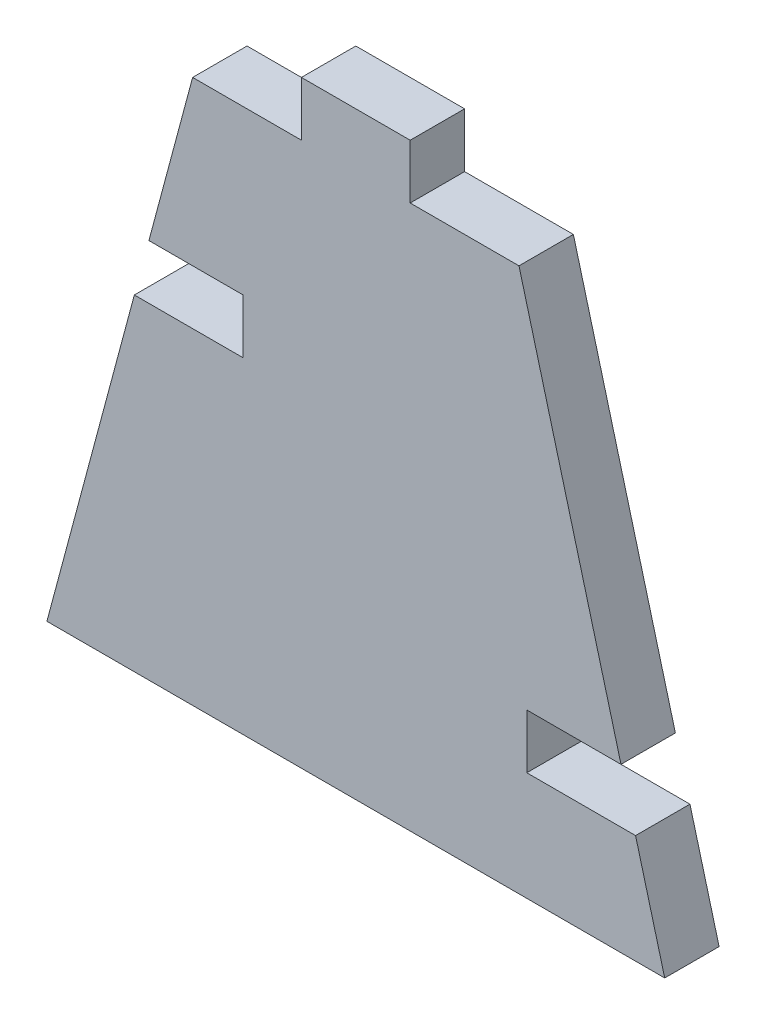
ISO-10303-21;
HEADER;
FILE_DESCRIPTION(('STEP AP214'),'2;1');
FILE_NAME('part.step','',(''),(''),'','','');
FILE_SCHEMA(('AUTOMOTIVE_DESIGN { 1 0 10303 214 1 1 1 1 }'));
ENDSEC;
DATA;
#1=APPLICATION_CONTEXT('core data for automotive mechanical design processes');
#2=APPLICATION_PROTOCOL_DEFINITION('international standard','automotive_design',2000,#1);
#3=PRODUCT_CONTEXT('',#1,'mechanical');
#4=PRODUCT('Part','Part','',(#3));
#5=PRODUCT_RELATED_PRODUCT_CATEGORY('part','',(#4));
#6=PRODUCT_DEFINITION_FORMATION('','',#4);
#7=PRODUCT_DEFINITION_CONTEXT('part definition',#1,'design');
#8=PRODUCT_DEFINITION('design','',#6,#7);
#9=PRODUCT_DEFINITION_SHAPE('','',#8);
#10=(LENGTH_UNIT() NAMED_UNIT(*) SI_UNIT(.MILLI.,.METRE.));
#11=(NAMED_UNIT(*) PLANE_ANGLE_UNIT() SI_UNIT($,.RADIAN.));
#12=(NAMED_UNIT(*) SI_UNIT($,.STERADIAN.) SOLID_ANGLE_UNIT());
#13=UNCERTAINTY_MEASURE_WITH_UNIT(LENGTH_MEASURE(1.E-05),#10,'distance_accuracy_value','');
#14=(GEOMETRIC_REPRESENTATION_CONTEXT(3) GLOBAL_UNCERTAINTY_ASSIGNED_CONTEXT((#13)) GLOBAL_UNIT_ASSIGNED_CONTEXT((#10,
#11,#12)) REPRESENTATION_CONTEXT('',''));
#15=CARTESIAN_POINT('',(0.,0.,0.));
#16=DIRECTION('',(0.,0.,1.));
#17=DIRECTION('',(1.,0.,0.));
#18=AXIS2_PLACEMENT_3D('',#15,#16,#17);
#19=CARTESIAN_POINT('',(0.,0.,5.));
#20=DIRECTION('',(0.965925826289069,-0.258819045102518,0.));
#21=DIRECTION('',(0.258819045102518,0.965925826289069,0.));
#22=AXIS2_PLACEMENT_3D('',#19,#20,#21);
#23=PLANE('',#22);
#24=DIRECTION('',(-0.258819045102518,-0.965925826289069,0.));
#25=VECTOR('',#24,1.);
#26=CARTESIAN_POINT('',(0.,0.,-5.));
#27=LINE('',#26,#25);
#28=CARTESIAN_POINT('',(16.0769515458672,60.,-5.));
#29=VERTEX_POINT('',#28);
#30=CARTESIAN_POINT('',(0.,0.,-5.));
#31=VERTEX_POINT('',#30);
#32=EDGE_CURVE('E181',#29,#31,#27,.T.);
#33=ORIENTED_EDGE('',*,*,#32,.T.);
#34=DIRECTION('',(0.,0.,-1.));
#35=VECTOR('',#34,1.);
#36=CARTESIAN_POINT('',(0.,0.,5.));
#37=LINE('',#36,#35);
#38=CARTESIAN_POINT('',(0.,0.,5.));
#39=VERTEX_POINT('',#38);
#40=EDGE_CURVE('E11',#39,#31,#37,.T.);
#41=ORIENTED_EDGE('',*,*,#40,.F.);
#42=DIRECTION('',(-0.258819045102518,-0.965925826289069,0.));
#43=VECTOR('',#42,1.);
#44=CARTESIAN_POINT('',(0.,0.,5.));
#45=LINE('',#44,#43);
#46=CARTESIAN_POINT('',(16.0769515458672,60.,5.));
#47=VERTEX_POINT('',#46);
#48=EDGE_CURVE('E213',#47,#39,#45,.T.);
#49=ORIENTED_EDGE('',*,*,#48,.F.);
#50=DIRECTION('',(0.,0.,-1.));
#51=VECTOR('',#50,1.);
#52=CARTESIAN_POINT('',(16.0769515458672,60.,5.));
#53=LINE('',#52,#51);
#54=EDGE_CURVE('E176',#47,#29,#53,.T.);
#55=ORIENTED_EDGE('',*,*,#54,.T.);
#56=EDGE_LOOP('',(#33,#41,#49,#55));
#57=FACE_BOUND('',#56,.T.);
#58=ADVANCED_FACE('F39',(#57),#23,.F.);
#59=CARTESIAN_POINT('',(0.,0.,5.));
#60=DIRECTION('',(0.,1.,0.));
#61=DIRECTION('',(0.,0.,1.));
#62=AXIS2_PLACEMENT_3D('',#59,#60,#61);
#63=PLANE('',#62);
#64=DIRECTION('',(1.,0.,0.));
#65=VECTOR('',#64,1.);
#66=CARTESIAN_POINT('',(0.,0.,-5.));
#67=LINE('',#66,#65);
#68=CARTESIAN_POINT('',(113.589838486224,0.,-5.));
#69=VERTEX_POINT('',#68);
#70=EDGE_CURVE('E187',#31,#69,#67,.T.);
#71=ORIENTED_EDGE('',*,*,#70,.T.);
#72=DIRECTION('',(0.,0.,-1.));
#73=VECTOR('',#72,1.);
#74=CARTESIAN_POINT('',(113.589838486224,0.,5.));
#75=LINE('',#74,#73);
#76=CARTESIAN_POINT('',(113.589838486224,0.,5.));
#77=VERTEX_POINT('',#76);
#78=EDGE_CURVE('E50',#77,#69,#75,.T.);
#79=ORIENTED_EDGE('',*,*,#78,.F.);
#80=DIRECTION('',(1.,0.,0.));
#81=VECTOR('',#80,1.);
#82=CARTESIAN_POINT('',(0.,0.,5.));
#83=LINE('',#82,#81);
#84=EDGE_CURVE('E125',#39,#77,#83,.T.);
#85=ORIENTED_EDGE('',*,*,#84,.F.);
#86=ORIENTED_EDGE('',*,*,#40,.T.);
#87=EDGE_LOOP('',(#71,#79,#85,#86));
#88=FACE_BOUND('',#87,.T.);
#89=ADVANCED_FACE('F313',(#88),#63,.F.);
#90=CARTESIAN_POINT('',(113.589838486224,0.,5.));
#91=DIRECTION('',(-0.965925826289069,-0.258819045102519,0.));
#92=DIRECTION('',(0.258819045102519,-0.965925826289069,0.));
#93=AXIS2_PLACEMENT_3D('',#90,#91,#92);
#94=PLANE('',#93);
#95=DIRECTION('',(-0.258819045102519,0.965925826289069,0.));
#96=VECTOR('',#95,1.);
#97=CARTESIAN_POINT('',(113.589838486224,0.,-5.));
#98=LINE('',#97,#96);
#99=CARTESIAN_POINT('',(108.230854637601,20.,-5.));
#100=VERTEX_POINT('',#99);
#101=EDGE_CURVE('E189',#69,#100,#98,.T.);
#102=ORIENTED_EDGE('',*,*,#101,.T.);
#103=DIRECTION('',(0.,0.,-1.));
#104=VECTOR('',#103,1.);
#105=CARTESIAN_POINT('',(108.230854637601,20.,5.));
#106=LINE('',#105,#104);
#107=CARTESIAN_POINT('',(108.230854637601,20.,5.));
#108=VERTEX_POINT('',#107);
#109=EDGE_CURVE('E241',#108,#100,#106,.T.);
#110=ORIENTED_EDGE('',*,*,#109,.F.);
#111=DIRECTION('',(-0.258819045102519,0.965925826289069,0.));
#112=VECTOR('',#111,1.);
#113=CARTESIAN_POINT('',(113.589838486224,0.,5.));
#114=LINE('',#113,#112);
#115=EDGE_CURVE('E252',#77,#108,#114,.T.);
#116=ORIENTED_EDGE('',*,*,#115,.F.);
#117=ORIENTED_EDGE('',*,*,#78,.T.);
#118=EDGE_LOOP('',(#102,#110,#116,#117));
#119=FACE_BOUND('',#118,.T.);
#120=ADVANCED_FACE('F248',(#119),#94,.F.);
#121=CARTESIAN_POINT('',(108.230854637601,20.,5.));
#122=DIRECTION('',(0.,-1.,0.));
#123=DIRECTION('',(1.,0.,0.));
#124=AXIS2_PLACEMENT_3D('',#121,#122,#123);
#125=PLANE('',#124);
#126=DIRECTION('',(-1.,0.,0.));
#127=VECTOR('',#126,1.);
#128=CARTESIAN_POINT('',(108.230854637601,20.,-5.));
#129=LINE('',#128,#127);
#130=CARTESIAN_POINT('',(88.2308546376015,20.,-5.));
#131=VERTEX_POINT('',#130);
#132=EDGE_CURVE('E188',#100,#131,#129,.T.);
#133=ORIENTED_EDGE('',*,*,#132,.T.);
#134=DIRECTION('',(0.,0.,-1.));
#135=VECTOR('',#134,1.);
#136=CARTESIAN_POINT('',(88.2308546376015,20.,5.));
#137=LINE('',#136,#135);
#138=CARTESIAN_POINT('',(88.2308546376015,20.,5.));
#139=VERTEX_POINT('',#138);
#140=EDGE_CURVE('E242',#139,#131,#137,.T.);
#141=ORIENTED_EDGE('',*,*,#140,.F.);
#142=DIRECTION('',(-1.,0.,0.));
#143=VECTOR('',#142,1.);
#144=CARTESIAN_POINT('',(108.230854637601,20.,5.));
#145=LINE('',#144,#143);
#146=EDGE_CURVE('E269',#108,#139,#145,.T.);
#147=ORIENTED_EDGE('',*,*,#146,.F.);
#148=ORIENTED_EDGE('',*,*,#109,.T.);
#149=EDGE_LOOP('',(#133,#141,#147,#148));
#150=FACE_BOUND('',#149,.T.);
#151=ADVANCED_FACE('F261',(#150),#125,.F.);
#152=CARTESIAN_POINT('',(88.2308546376015,20.,5.));
#153=DIRECTION('',(-1.,0.,0.));
#154=DIRECTION('',(0.,0.,1.));
#155=AXIS2_PLACEMENT_3D('',#152,#153,#154);
#156=PLANE('',#155);
#157=DIRECTION('',(0.,1.,0.));
#158=VECTOR('',#157,1.);
#159=CARTESIAN_POINT('',(88.2308546376015,20.,-5.));
#160=LINE('',#159,#158);
#161=CARTESIAN_POINT('',(88.2308546376015,30.,-5.));
#162=VERTEX_POINT('',#161);
#163=EDGE_CURVE('E195',#131,#162,#160,.T.);
#164=ORIENTED_EDGE('',*,*,#163,.T.);
#165=DIRECTION('',(0.,0.,-1.));
#166=VECTOR('',#165,1.);
#167=CARTESIAN_POINT('',(88.2308546376015,30.,5.));
#168=LINE('',#167,#166);
#169=CARTESIAN_POINT('',(88.2308546376015,30.,5.));
#170=VERTEX_POINT('',#169);
#171=EDGE_CURVE('E236',#170,#162,#168,.T.);
#172=ORIENTED_EDGE('',*,*,#171,.F.);
#173=DIRECTION('',(0.,1.,0.));
#174=VECTOR('',#173,1.);
#175=CARTESIAN_POINT('',(88.2308546376015,20.,5.));
#176=LINE('',#175,#174);
#177=EDGE_CURVE('E270',#139,#170,#176,.T.);
#178=ORIENTED_EDGE('',*,*,#177,.F.);
#179=ORIENTED_EDGE('',*,*,#140,.T.);
#180=EDGE_LOOP('',(#164,#172,#178,#179));
#181=FACE_BOUND('',#180,.T.);
#182=ADVANCED_FACE('F264',(#181),#156,.F.);
#183=CARTESIAN_POINT('',(88.2308546376015,30.,5.));
#184=DIRECTION('',(0.,1.,0.));
#185=DIRECTION('',(0.,0.,1.));
#186=AXIS2_PLACEMENT_3D('',#183,#184,#185);
#187=PLANE('',#186);
#188=DIRECTION('',(1.,0.,0.));
#189=VECTOR('',#188,1.);
#190=CARTESIAN_POINT('',(88.2308546376015,30.,-5.));
#191=LINE('',#190,#189);
#192=CARTESIAN_POINT('',(105.55136271329,30.,-5.));
#193=VERTEX_POINT('',#192);
#194=EDGE_CURVE('E191',#162,#193,#191,.T.);
#195=ORIENTED_EDGE('',*,*,#194,.T.);
#196=DIRECTION('',(0.,0.,-1.));
#197=VECTOR('',#196,1.);
#198=CARTESIAN_POINT('',(105.55136271329,30.,5.));
#199=LINE('',#198,#197);
#200=CARTESIAN_POINT('',(105.55136271329,30.,5.));
#201=VERTEX_POINT('',#200);
#202=EDGE_CURVE('E233',#201,#193,#199,.T.);
#203=ORIENTED_EDGE('',*,*,#202,.F.);
#204=DIRECTION('',(1.,0.,0.));
#205=VECTOR('',#204,1.);
#206=CARTESIAN_POINT('',(88.2308546376015,30.,5.));
#207=LINE('',#206,#205);
#208=EDGE_CURVE('E267',#170,#201,#207,.T.);
#209=ORIENTED_EDGE('',*,*,#208,.F.);
#210=ORIENTED_EDGE('',*,*,#171,.T.);
#211=EDGE_LOOP('',(#195,#203,#209,#210));
#212=FACE_BOUND('',#211,.T.);
#213=ADVANCED_FACE('F322',(#212),#187,.F.);
#214=CARTESIAN_POINT('',(105.55136271329,30.,5.));
#215=DIRECTION('',(-0.965925826289069,-0.258819045102517,0.));
#216=DIRECTION('',(0.258819045102517,-0.965925826289069,0.));
#217=AXIS2_PLACEMENT_3D('',#214,#215,#216);
#218=PLANE('',#217);
#219=DIRECTION('',(-0.258819045102517,0.965925826289069,0.));
#220=VECTOR('',#219,1.);
#221=CARTESIAN_POINT('',(105.55136271329,30.,-5.));
#222=LINE('',#221,#220);
#223=CARTESIAN_POINT('',(86.794919243112,100.,-5.));
#224=VERTEX_POINT('',#223);
#225=EDGE_CURVE('E198',#193,#224,#222,.T.);
#226=ORIENTED_EDGE('',*,*,#225,.T.);
#227=DIRECTION('',(0.,0.,-1.));
#228=VECTOR('',#227,1.);
#229=CARTESIAN_POINT('',(86.794919243112,100.,5.));
#230=LINE('',#229,#228);
#231=CARTESIAN_POINT('',(86.794919243112,100.,5.));
#232=VERTEX_POINT('',#231);
#233=EDGE_CURVE('E235',#232,#224,#230,.T.);
#234=ORIENTED_EDGE('',*,*,#233,.F.);
#235=DIRECTION('',(-0.258819045102517,0.965925826289069,0.));
#236=VECTOR('',#235,1.);
#237=CARTESIAN_POINT('',(105.55136271329,30.,5.));
#238=LINE('',#237,#236);
#239=EDGE_CURVE('E275',#201,#232,#238,.T.);
#240=ORIENTED_EDGE('',*,*,#239,.F.);
#241=ORIENTED_EDGE('',*,*,#202,.T.);
#242=EDGE_LOOP('',(#226,#234,#240,#241));
#243=FACE_BOUND('',#242,.T.);
#244=ADVANCED_FACE('F330',(#243),#218,.F.);
#245=CARTESIAN_POINT('',(86.794919243112,100.,5.));
#246=DIRECTION('',(0.,-1.,0.));
#247=DIRECTION('',(0.,0.,-1.));
#248=AXIS2_PLACEMENT_3D('',#245,#246,#247);
#249=PLANE('',#248);
#250=DIRECTION('',(-1.,0.,0.));
#251=VECTOR('',#250,1.);
#252=CARTESIAN_POINT('',(86.794919243112,100.,-5.));
#253=LINE('',#252,#251);
#254=CARTESIAN_POINT('',(66.7949192431119,100.,-5.));
#255=VERTEX_POINT('',#254);
#256=EDGE_CURVE('E196',#224,#255,#253,.T.);
#257=ORIENTED_EDGE('',*,*,#256,.T.);
#258=DIRECTION('',(0.,0.,-1.));
#259=VECTOR('',#258,1.);
#260=CARTESIAN_POINT('',(66.7949192431119,100.,5.));
#261=LINE('',#260,#259);
#262=CARTESIAN_POINT('',(66.7949192431119,100.,5.));
#263=VERTEX_POINT('',#262);
#264=EDGE_CURVE('E226',#263,#255,#261,.T.);
#265=ORIENTED_EDGE('',*,*,#264,.F.);
#266=DIRECTION('',(-1.,0.,0.));
#267=VECTOR('',#266,1.);
#268=CARTESIAN_POINT('',(86.794919243112,100.,5.));
#269=LINE('',#268,#267);
#270=EDGE_CURVE('E279',#232,#263,#269,.T.);
#271=ORIENTED_EDGE('',*,*,#270,.F.);
#272=ORIENTED_EDGE('',*,*,#233,.T.);
#273=EDGE_LOOP('',(#257,#265,#271,#272));
#274=FACE_BOUND('',#273,.T.);
#275=ADVANCED_FACE('F332',(#274),#249,.F.);
#276=CARTESIAN_POINT('',(66.7949192431119,100.,5.));
#277=DIRECTION('',(-1.,0.,0.));
#278=DIRECTION('',(0.,-1.,0.));
#279=AXIS2_PLACEMENT_3D('',#276,#277,#278);
#280=PLANE('',#279);
#281=DIRECTION('',(0.,1.,0.));
#282=VECTOR('',#281,1.);
#283=CARTESIAN_POINT('',(66.7949192431119,100.,-5.));
#284=LINE('',#283,#282);
#285=CARTESIAN_POINT('',(66.7949192431119,110.,-5.));
#286=VERTEX_POINT('',#285);
#287=EDGE_CURVE('E199',#255,#286,#284,.T.);
#288=ORIENTED_EDGE('',*,*,#287,.T.);
#289=DIRECTION('',(0.,0.,-1.));
#290=VECTOR('',#289,1.);
#291=CARTESIAN_POINT('',(66.7949192431119,110.,5.));
#292=LINE('',#291,#290);
#293=CARTESIAN_POINT('',(66.7949192431119,110.,5.));
#294=VERTEX_POINT('',#293);
#295=EDGE_CURVE('E227',#294,#286,#292,.T.);
#296=ORIENTED_EDGE('',*,*,#295,.F.);
#297=DIRECTION('',(0.,1.,0.));
#298=VECTOR('',#297,1.);
#299=CARTESIAN_POINT('',(66.7949192431119,100.,5.));
#300=LINE('',#299,#298);
#301=EDGE_CURVE('E278',#263,#294,#300,.T.);
#302=ORIENTED_EDGE('',*,*,#301,.F.);
#303=ORIENTED_EDGE('',*,*,#264,.T.);
#304=EDGE_LOOP('',(#288,#296,#302,#303));
#305=FACE_BOUND('',#304,.T.);
#306=ADVANCED_FACE('F333',(#305),#280,.F.);
#307=CARTESIAN_POINT('',(46.7949192431119,110.,5.));
#308=DIRECTION('',(0.,-1.,0.));
#309=DIRECTION('',(0.,0.,-1.));
#310=AXIS2_PLACEMENT_3D('',#307,#308,#309);
#311=PLANE('',#310);
#312=DIRECTION('',(-1.,0.,0.));
#313=VECTOR('',#312,1.);
#314=CARTESIAN_POINT('',(46.7949192431119,110.,-5.));
#315=LINE('',#314,#313);
#316=CARTESIAN_POINT('',(46.7949192431119,110.,-5.));
#317=VERTEX_POINT('',#316);
#318=EDGE_CURVE('E205',#286,#317,#315,.T.);
#319=ORIENTED_EDGE('',*,*,#318,.T.);
#320=DIRECTION('',(0.,0.,-1.));
#321=VECTOR('',#320,1.);
#322=CARTESIAN_POINT('',(46.7949192431119,110.,5.));
#323=LINE('',#322,#321);
#324=CARTESIAN_POINT('',(46.7949192431119,110.,5.));
#325=VERTEX_POINT('',#324);
#326=EDGE_CURVE('E224',#325,#317,#323,.T.);
#327=ORIENTED_EDGE('',*,*,#326,.F.);
#328=DIRECTION('',(-1.,0.,0.));
#329=VECTOR('',#328,1.);
#330=CARTESIAN_POINT('',(46.7949192431119,110.,5.));
#331=LINE('',#330,#329);
#332=EDGE_CURVE('E285',#294,#325,#331,.T.);
#333=ORIENTED_EDGE('',*,*,#332,.F.);
#334=ORIENTED_EDGE('',*,*,#295,.T.);
#335=EDGE_LOOP('',(#319,#327,#333,#334));
#336=FACE_BOUND('',#335,.T.);
#337=ADVANCED_FACE('F336',(#336),#311,.F.);
#338=CARTESIAN_POINT('',(46.7949192431119,100.,5.));
#339=DIRECTION('',(1.,0.,0.));
#340=DIRECTION('',(0.,1.,0.));
#341=AXIS2_PLACEMENT_3D('',#338,#339,#340);
#342=PLANE('',#341);
#343=DIRECTION('',(0.,-1.,0.));
#344=VECTOR('',#343,1.);
#345=CARTESIAN_POINT('',(46.7949192431119,100.,-5.));
#346=LINE('',#345,#344);
#347=CARTESIAN_POINT('',(46.7949192431119,100.,-5.));
#348=VERTEX_POINT('',#347);
#349=EDGE_CURVE('E204',#317,#348,#346,.T.);
#350=ORIENTED_EDGE('',*,*,#349,.T.);
#351=DIRECTION('',(0.,0.,-1.));
#352=VECTOR('',#351,1.);
#353=CARTESIAN_POINT('',(46.7949192431119,100.,5.));
#354=LINE('',#353,#352);
#355=CARTESIAN_POINT('',(46.7949192431119,100.,5.));
#356=VERTEX_POINT('',#355);
#357=EDGE_CURVE('E219',#356,#348,#354,.T.);
#358=ORIENTED_EDGE('',*,*,#357,.F.);
#359=DIRECTION('',(0.,-1.,0.));
#360=VECTOR('',#359,1.);
#361=CARTESIAN_POINT('',(46.7949192431119,100.,5.));
#362=LINE('',#361,#360);
#363=EDGE_CURVE('E281',#325,#356,#362,.T.);
#364=ORIENTED_EDGE('',*,*,#363,.F.);
#365=ORIENTED_EDGE('',*,*,#326,.T.);
#366=EDGE_LOOP('',(#350,#358,#364,#365));
#367=FACE_BOUND('',#366,.T.);
#368=ADVANCED_FACE('F344',(#367),#342,.F.);
#369=CARTESIAN_POINT('',(26.7949192431119,100.,5.));
#370=DIRECTION('',(0.,-1.,0.));
#371=DIRECTION('',(0.,0.,-1.));
#372=AXIS2_PLACEMENT_3D('',#369,#370,#371);
#373=PLANE('',#372);
#374=DIRECTION('',(-1.,0.,0.));
#375=VECTOR('',#374,1.);
#376=CARTESIAN_POINT('',(26.7949192431119,100.,-5.));
#377=LINE('',#376,#375);
#378=CARTESIAN_POINT('',(26.7949192431119,100.,-5.));
#379=VERTEX_POINT('',#378);
#380=EDGE_CURVE('E206',#348,#379,#377,.T.);
#381=ORIENTED_EDGE('',*,*,#380,.T.);
#382=DIRECTION('',(0.,0.,-1.));
#383=VECTOR('',#382,1.);
#384=CARTESIAN_POINT('',(26.7949192431119,100.,5.));
#385=LINE('',#384,#383);
#386=CARTESIAN_POINT('',(26.7949192431119,100.,5.));
#387=VERTEX_POINT('',#386);
#388=EDGE_CURVE('E220',#387,#379,#385,.T.);
#389=ORIENTED_EDGE('',*,*,#388,.F.);
#390=DIRECTION('',(-1.,0.,0.));
#391=VECTOR('',#390,1.);
#392=CARTESIAN_POINT('',(26.7949192431119,100.,5.));
#393=LINE('',#392,#391);
#394=EDGE_CURVE('E287',#356,#387,#393,.T.);
#395=ORIENTED_EDGE('',*,*,#394,.F.);
#396=ORIENTED_EDGE('',*,*,#357,.T.);
#397=EDGE_LOOP('',(#381,#389,#395,#396));
#398=FACE_BOUND('',#397,.T.);
#399=ADVANCED_FACE('F295',(#398),#373,.F.);
#400=CARTESIAN_POINT('',(18.7564434701784,70.,5.));
#401=DIRECTION('',(0.965925826289069,-0.258819045102518,0.));
#402=DIRECTION('',(0.258819045102518,0.965925826289069,0.));
#403=AXIS2_PLACEMENT_3D('',#400,#401,#402);
#404=PLANE('',#403);
#405=DIRECTION('',(-0.258819045102518,-0.965925826289069,0.));
#406=VECTOR('',#405,1.);
#407=CARTESIAN_POINT('',(18.7564434701784,70.,-5.));
#408=LINE('',#407,#406);
#409=CARTESIAN_POINT('',(18.7564434701784,70.,-5.));
#410=VERTEX_POINT('',#409);
#411=EDGE_CURVE('E208',#379,#410,#408,.T.);
#412=ORIENTED_EDGE('',*,*,#411,.T.);
#413=DIRECTION('',(0.,0.,-1.));
#414=VECTOR('',#413,1.);
#415=CARTESIAN_POINT('',(18.7564434701784,70.,5.));
#416=LINE('',#415,#414);
#417=CARTESIAN_POINT('',(18.7564434701784,70.,5.));
#418=VERTEX_POINT('',#417);
#419=EDGE_CURVE('E171',#418,#410,#416,.T.);
#420=ORIENTED_EDGE('',*,*,#419,.F.);
#421=DIRECTION('',(-0.258819045102518,-0.965925826289069,0.));
#422=VECTOR('',#421,1.);
#423=CARTESIAN_POINT('',(18.7564434701784,70.,5.));
#424=LINE('',#423,#422);
#425=EDGE_CURVE('E164',#387,#418,#424,.T.);
#426=ORIENTED_EDGE('',*,*,#425,.F.);
#427=ORIENTED_EDGE('',*,*,#388,.T.);
#428=EDGE_LOOP('',(#412,#420,#426,#427));
#429=FACE_BOUND('',#428,.T.);
#430=ADVANCED_FACE('F297',(#429),#404,.F.);
#431=CARTESIAN_POINT('',(36.0769515458672,70.,5.));
#432=DIRECTION('',(0.,1.,0.));
#433=DIRECTION('',(-1.,0.,0.));
#434=AXIS2_PLACEMENT_3D('',#431,#432,#433);
#435=PLANE('',#434);
#436=DIRECTION('',(1.,0.,0.));
#437=VECTOR('',#436,1.);
#438=CARTESIAN_POINT('',(36.0769515458672,70.,-5.));
#439=LINE('',#438,#437);
#440=CARTESIAN_POINT('',(36.0769515458672,70.,-5.));
#441=VERTEX_POINT('',#440);
#442=EDGE_CURVE('E174',#410,#441,#439,.T.);
#443=ORIENTED_EDGE('',*,*,#442,.T.);
#444=DIRECTION('',(0.,0.,-1.));
#445=VECTOR('',#444,1.);
#446=CARTESIAN_POINT('',(36.0769515458672,70.,5.));
#447=LINE('',#446,#445);
#448=CARTESIAN_POINT('',(36.0769515458672,70.,5.));
#449=VERTEX_POINT('',#448);
#450=EDGE_CURVE('E168',#449,#441,#447,.T.);
#451=ORIENTED_EDGE('',*,*,#450,.F.);
#452=DIRECTION('',(1.,0.,0.));
#453=VECTOR('',#452,1.);
#454=CARTESIAN_POINT('',(36.0769515458672,70.,5.));
#455=LINE('',#454,#453);
#456=EDGE_CURVE('E157',#418,#449,#455,.T.);
#457=ORIENTED_EDGE('',*,*,#456,.F.);
#458=ORIENTED_EDGE('',*,*,#419,.T.);
#459=EDGE_LOOP('',(#443,#451,#457,#458));
#460=FACE_BOUND('',#459,.T.);
#461=ADVANCED_FACE('F172',(#460),#435,.F.);
#462=CARTESIAN_POINT('',(36.0769515458672,60.,5.));
#463=DIRECTION('',(1.,0.,0.));
#464=DIRECTION('',(0.,0.,-1.));
#465=AXIS2_PLACEMENT_3D('',#462,#463,#464);
#466=PLANE('',#465);
#467=DIRECTION('',(0.,-1.,0.));
#468=VECTOR('',#467,1.);
#469=CARTESIAN_POINT('',(36.0769515458672,60.,-5.));
#470=LINE('',#469,#468);
#471=CARTESIAN_POINT('',(36.0769515458672,60.,-5.));
#472=VERTEX_POINT('',#471);
#473=EDGE_CURVE('E107',#441,#472,#470,.T.);
#474=ORIENTED_EDGE('',*,*,#473,.T.);
#475=DIRECTION('',(0.,0.,-1.));
#476=VECTOR('',#475,1.);
#477=CARTESIAN_POINT('',(36.0769515458672,60.,5.));
#478=LINE('',#477,#476);
#479=CARTESIAN_POINT('',(36.0769515458672,60.,5.));
#480=VERTEX_POINT('',#479);
#481=EDGE_CURVE('E173',#480,#472,#478,.T.);
#482=ORIENTED_EDGE('',*,*,#481,.F.);
#483=DIRECTION('',(0.,-1.,0.));
#484=VECTOR('',#483,1.);
#485=CARTESIAN_POINT('',(36.0769515458672,60.,5.));
#486=LINE('',#485,#484);
#487=EDGE_CURVE('E162',#449,#480,#486,.T.);
#488=ORIENTED_EDGE('',*,*,#487,.F.);
#489=ORIENTED_EDGE('',*,*,#450,.T.);
#490=EDGE_LOOP('',(#474,#482,#488,#489));
#491=FACE_BOUND('',#490,.T.);
#492=ADVANCED_FACE('F180',(#491),#466,.F.);
#493=CARTESIAN_POINT('',(16.0769515458672,60.,5.));
#494=DIRECTION('',(0.,-1.,0.));
#495=DIRECTION('',(0.,0.,-1.));
#496=AXIS2_PLACEMENT_3D('',#493,#494,#495);
#497=PLANE('',#496);
#498=DIRECTION('',(-1.,0.,0.));
#499=VECTOR('',#498,1.);
#500=CARTESIAN_POINT('',(16.0769515458672,60.,-5.));
#501=LINE('',#500,#499);
#502=EDGE_CURVE('E111',#472,#29,#501,.T.);
#503=ORIENTED_EDGE('',*,*,#502,.T.);
#504=ORIENTED_EDGE('',*,*,#54,.F.);
#505=DIRECTION('',(-1.,0.,0.));
#506=VECTOR('',#505,1.);
#507=CARTESIAN_POINT('',(16.0769515458672,60.,5.));
#508=LINE('',#507,#506);
#509=EDGE_CURVE('E54',#480,#47,#508,.T.);
#510=ORIENTED_EDGE('',*,*,#509,.F.);
#511=ORIENTED_EDGE('',*,*,#481,.T.);
#512=EDGE_LOOP('',(#503,#504,#510,#511));
#513=FACE_BOUND('',#512,.T.);
#514=ADVANCED_FACE('F298',(#513),#497,.F.);
#515=CARTESIAN_POINT('',(0.,0.,5.));
#516=DIRECTION('',(0.,0.,-1.));
#517=DIRECTION('',(-1.,0.,0.));
#518=AXIS2_PLACEMENT_3D('',#515,#516,#517);
#519=PLANE('',#518);
#520=ORIENTED_EDGE('',*,*,#48,.T.);
#521=ORIENTED_EDGE('',*,*,#84,.T.);
#522=ORIENTED_EDGE('',*,*,#115,.T.);
#523=ORIENTED_EDGE('',*,*,#146,.T.);
#524=ORIENTED_EDGE('',*,*,#177,.T.);
#525=ORIENTED_EDGE('',*,*,#208,.T.);
#526=ORIENTED_EDGE('',*,*,#239,.T.);
#527=ORIENTED_EDGE('',*,*,#270,.T.);
#528=ORIENTED_EDGE('',*,*,#301,.T.);
#529=ORIENTED_EDGE('',*,*,#332,.T.);
#530=ORIENTED_EDGE('',*,*,#363,.T.);
#531=ORIENTED_EDGE('',*,*,#394,.T.);
#532=ORIENTED_EDGE('',*,*,#425,.T.);
#533=ORIENTED_EDGE('',*,*,#456,.T.);
#534=ORIENTED_EDGE('',*,*,#487,.T.);
#535=ORIENTED_EDGE('',*,*,#509,.T.);
#536=EDGE_LOOP('',(#520,#521,#522,#523,#524,#525,#526,#527,#528,#529,#530,#531,#532,#533,#534,#535));
#537=FACE_BOUND('',#536,.T.);
#538=ADVANCED_FACE('F161',(#537),#519,.F.);
#539=CARTESIAN_POINT('',(0.,0.,-5.));
#540=DIRECTION('',(0.,0.,-1.));
#541=DIRECTION('',(-1.,0.,0.));
#542=AXIS2_PLACEMENT_3D('',#539,#540,#541);
#543=PLANE('',#542);
#544=ORIENTED_EDGE('',*,*,#32,.F.);
#545=ORIENTED_EDGE('',*,*,#502,.F.);
#546=ORIENTED_EDGE('',*,*,#473,.F.);
#547=ORIENTED_EDGE('',*,*,#442,.F.);
#548=ORIENTED_EDGE('',*,*,#411,.F.);
#549=ORIENTED_EDGE('',*,*,#380,.F.);
#550=ORIENTED_EDGE('',*,*,#349,.F.);
#551=ORIENTED_EDGE('',*,*,#318,.F.);
#552=ORIENTED_EDGE('',*,*,#287,.F.);
#553=ORIENTED_EDGE('',*,*,#256,.F.);
#554=ORIENTED_EDGE('',*,*,#225,.F.);
#555=ORIENTED_EDGE('',*,*,#194,.F.);
#556=ORIENTED_EDGE('',*,*,#163,.F.);
#557=ORIENTED_EDGE('',*,*,#132,.F.);
#558=ORIENTED_EDGE('',*,*,#101,.F.);
#559=ORIENTED_EDGE('',*,*,#70,.F.);
#560=EDGE_LOOP('',(#544,#545,#546,#547,#548,#549,#550,#551,#552,#553,#554,#555,#556,#557,#558,#559));
#561=FACE_BOUND('',#560,.T.);
#562=ADVANCED_FACE('F258',(#561),#543,.T.);
#563=CLOSED_SHELL('',(#58,#89,#120,#151,#182,#213,#244,#275,#306,#337,#368,#399,#430,#461,#492,
#514,#538,#562));
#564=MANIFOLD_SOLID_BREP('B2',#563);
#565=ADVANCED_BREP_SHAPE_REPRESENTATION('',(#18,#564),#14);
#566=SHAPE_DEFINITION_REPRESENTATION(#9,#565);
ENDSEC;
END-ISO-10303-21;
